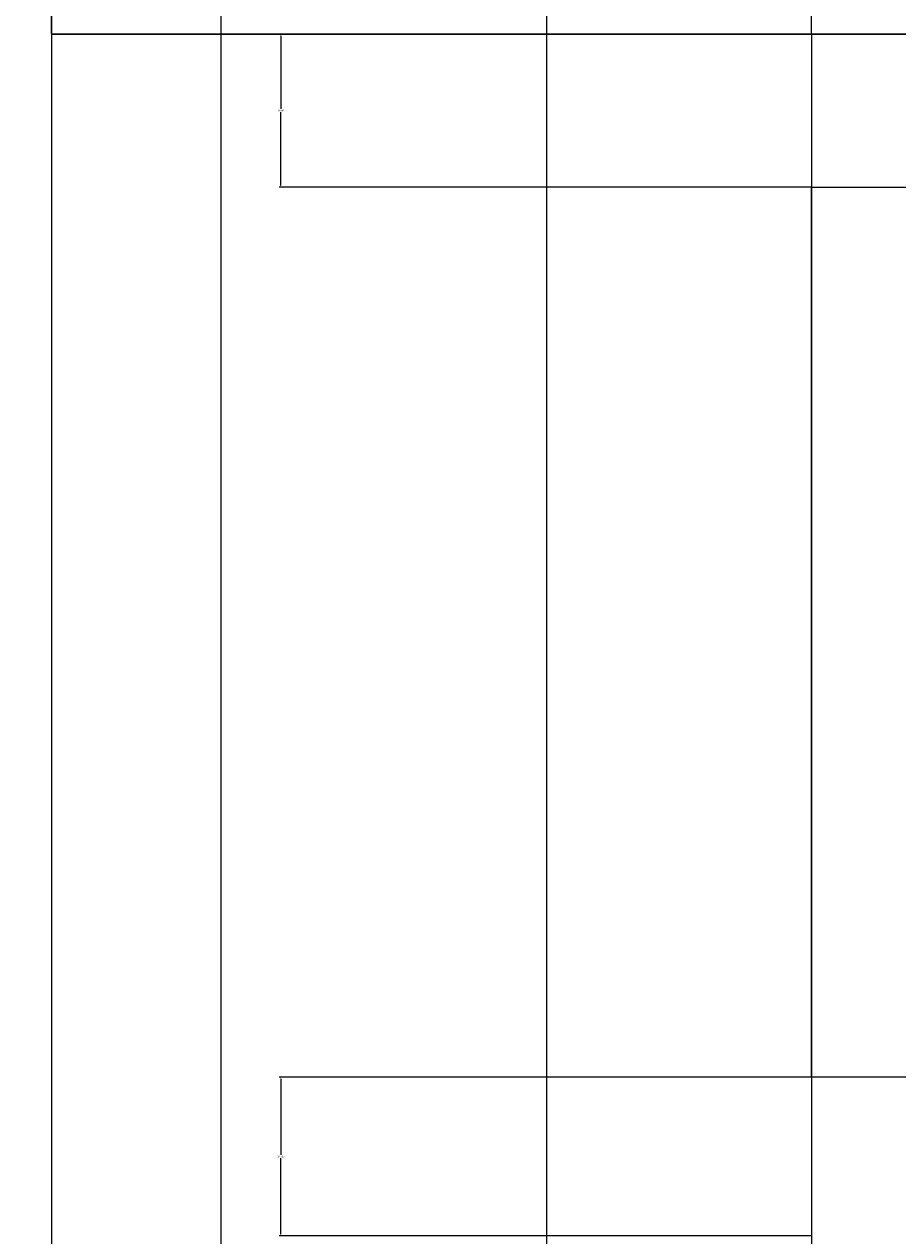
# Model space of a CAD drawing. Units: inches. Extents: x -46 to 1145, y -527 to 760.
# Tile 10 of 57: x 187 to 283, y -172 to -38. Entities that reach past the tile are written whole.
import ezdxf

# ---------------------------------------------------------------- set-up
doc = ezdxf.new("R2010")
doc.units = ezdxf.units.IN
doc.header["$MEASUREMENT"] = 0
for name, color, linetype, lineweight in [('A-ANNO-DIMS', 2, 'Continuous', 18), ('C-PKNG', 8, 'Continuous', 18), ('C-ROAD', 9, 'Continuous', 18), ('C-SITE', 7, 'Continuous', 30)]:
    doc.layers.add(name, color=color, linetype=linetype, lineweight=lineweight)
doc.styles.get("Standard").update_dxf_attribs({"font": 'arial.ttf'})
doc.dimstyles.get("Standard").update_dxf_attribs({"dimtxt": 0.18, "dimasz": 0.18, "dimexe": 0.18, "dimexo": 0.0625, "dimgap": 0.09, "dimtad": 0, "dimtih": 1, "dimtoh": 1, "dimdec": 0, "dimzin": 0, "dimdsep": 46, "dimlunit": 3, "dimtxsty": 'Standard', "dimcen": 0.09, "dimadec": 0, "dimazin": 0, "dimtfac": 1, "dimtdec": 0, "dimtofl": 0, "dimtmove": 0, "dimatfit": 3, "dimfxl": 1, "dimtolj": 1, "dimtzin": 0, "dimarcsym": 0})

# ---------------------------------------------------------------- blocks, each defined once
blk = doc.blocks.new('*D693')
at = {"layer": 'A-ANNO-DIMS', "color": 0, "lineweight": -2, "transparency": 16777216}
for p, q in [((189.56, -39.42), (189.56, 19.3)), ((189.74, 19.12), (231.15, 19.12)), ((273.34, 19.12), (231.93, 19.12)), ((273.52, -39.42), (273.52, 19.3))]:
    blk.add_line(p, q, dxfattribs=at)
at = {"layer": 'A-ANNO-DIMS', "color": 0, "transparency": 16777216}
for points in [[(189.74, 19.15), (189.74, 19.09), (189.56, 19.12)], [(273.34, 19.15), (273.34, 19.09), (273.52, 19.12)]]:
    blk.add_solid(points, dxfattribs=at)
at = {"layer": 'Defpoints', "color": 0, "transparency": 16777216}
for p in [(273.52, 19.12), (189.56, -39.48), (273.52, -39.48)]:
    blk.add_point(p, dxfattribs=at)
at = {"layer": 'A-ANNO-DIMS', "color": 0, "transparency": 16777216, "insert": (231.54, 19.12), "char_height": 0.18, "attachment_point": 5}
blk.add_mtext('\\A1;83.95', dxfattribs=at)
blk = doc.blocks.new('*D695')
at = {"layer": 'A-ANNO-DIMS', "color": 0, "lineweight": -2, "transparency": 16777216}
for p, q in [((208.27, 221.46), (208.27, -527.26)), ((244.27, 221.46), (244.27, -527.26)), ((208.45, -527.08), (226.05, -527.08)), ((244.09, -527.08), (226.49, -527.08))]:
    blk.add_line(p, q, dxfattribs=at)
at = {"layer": 'A-ANNO-DIMS', "color": 0, "transparency": 16777216}
for points in [[(208.45, -527.05), (208.45, -527.11), (208.27, -527.08)], [(244.09, -527.05), (244.09, -527.11), (244.27, -527.08)]]:
    blk.add_solid(points, dxfattribs=at)
at = {"layer": 'Defpoints', "color": 0, "transparency": 16777216}
for p in [(208.27, 221.52), (244.27, 221.52), (244.27, -527.08)]:
    blk.add_point(p, dxfattribs=at)
at = {"layer": 'A-ANNO-DIMS', "color": 0, "transparency": 16777216, "insert": (226.27, -527.08), "char_height": 0.18, "attachment_point": 5}
blk.add_mtext('\\A1;36', dxfattribs=at)
blk = doc.blocks.new('*D701')
at = {"layer": 'A-ANNO-DIMS', "color": 0, "lineweight": -2, "transparency": 16777216}
for p, q in [((273.45, -154.67), (214.74, -154.67)), ((214.92, -154.85), (214.92, -163.24)), ((214.92, -172), (214.92, -163.61)), ((273.45, -172.18), (214.74, -172.18))]:
    blk.add_line(p, q, dxfattribs=at)
at = {"layer": 'A-ANNO-DIMS', "color": 0, "transparency": 16777216}
for points in [[(214.89, -154.85), (214.95, -154.85), (214.92, -154.67)], [(214.89, -172), (214.95, -172), (214.92, -172.18)]]:
    blk.add_solid(points, dxfattribs=at)
at = {"layer": 'Defpoints', "color": 0, "transparency": 16777216}
for p in [(214.92, -154.67), (273.52, -154.67), (273.52, -172.18)]:
    blk.add_point(p, dxfattribs=at)
at = {"layer": 'A-ANNO-DIMS', "color": 0, "transparency": 16777216, "insert": (214.92, -163.42), "char_height": 0.18, "attachment_point": 5}
blk.add_mtext('\\A1;17.513', dxfattribs=at)
blk = doc.blocks.new('*D702')
at = {"layer": 'A-ANNO-DIMS', "color": 0, "lineweight": -2, "transparency": 16777216}
for p, q in [((189.63, -39.48), (1145.34, -39.48)), ((1145.16, -39.66), (1145.16, -249.3)), ((1145.16, -459.3), (1145.16, -249.66)), ((183.63, -459.48), (1145.34, -459.48))]:
    blk.add_line(p, q, dxfattribs=at)
at = {"layer": 'A-ANNO-DIMS', "color": 0, "transparency": 16777216}
for points in [[(1145.13, -39.66), (1145.19, -39.66), (1145.16, -39.48)], [(1145.13, -459.3), (1145.19, -459.3), (1145.16, -459.48)]]:
    blk.add_solid(points, dxfattribs=at)
at = {"layer": 'Defpoints', "color": 0, "transparency": 16777216}
for p in [(189.56, -39.48), (1145.16, -39.48), (183.56, -459.48)]:
    blk.add_point(p, dxfattribs=at)
at = {"layer": 'A-ANNO-DIMS', "color": 0, "transparency": 16777216, "insert": (1145.16, -249.48), "char_height": 0.18, "attachment_point": 5}
blk.add_mtext('\\A1;420', dxfattribs=at)
blk = doc.blocks.new('*D703')
at = {"layer": 'A-ANNO-DIMS', "color": 0, "lineweight": -2, "transparency": 16777216}
for p, q in [((273.45, -39.48), (214.74, -39.48)), ((214.92, -39.66), (214.92, -47.74)), ((214.92, -56.19), (214.92, -48.11)), ((273.45, -56.37), (214.74, -56.37))]:
    blk.add_line(p, q, dxfattribs=at)
at = {"layer": 'A-ANNO-DIMS', "color": 0, "transparency": 16777216}
for points in [[(214.89, -39.66), (214.95, -39.66), (214.92, -39.48)], [(214.89, -56.19), (214.95, -56.19), (214.92, -56.37)]]:
    blk.add_solid(points, dxfattribs=at)
at = {"layer": 'Defpoints', "color": 0, "transparency": 16777216}
for p in [(214.92, -39.48), (273.52, -39.48), (273.52, -56.37)]:
    blk.add_point(p, dxfattribs=at)
at = {"layer": 'A-ANNO-DIMS', "color": 0, "transparency": 16777216, "insert": (214.92, -47.93), "char_height": 0.18, "attachment_point": 5}
blk.add_mtext('\\A1;16.888', dxfattribs=at)

msp = doc.modelspace()

# ---------------------------------------------------------------- linework, layer by layer
at = {"layer": 'C-PKNG'}
msp.add_line((273.5156, -39.4824), (273.5156, -459.4824), dxfattribs=at)
msp.add_lwpolyline([(501.7297, -154.6684), (273.5156, -154.6684), (273.5156, -56.3706), (501.7297, -56.3706)], close=True, dxfattribs=at)
at = {"layer": 'C-ROAD'}
msp.add_line((189.5637, 221.5176), (189.5637, -468.4824), dxfattribs=at)
at = {"layer": 'C-SITE'}
msp.add_line((590.0637, -39.4824), (189.5637, -39.4824), dxfattribs=at)

# ---------------------------------------------------------------- dimensions: what is measured, and where the dimension line sits
at = {"layer": 'A-ANNO-DIMS'}
for base, p1, p2, override, picture, middle in [((244.2731, -527.0824), (208.2731, 221.5176), (244.2731, 221.5176), {"dimdec": 0, "dimlfac": 1, "dimrnd": 0, "dimzin": 0, "dimdsep": 46, "dimlunit": 2}, '*D695', (226.2731, -527.0824)), ((273.5156, 19.1176), (189.5637, -39.4824), (273.5156, -39.4824), {"dimdec": 2, "dimlfac": 1, "dimrnd": 0, "dimzin": 0, "dimdsep": 46, "dimlunit": 2}, '*D693', (231.5397, 19.1176))]:
    dim = msp.add_linear_dim(base=base, p1=p1, p2=p2, dimstyle='Standard', override=override, dxfattribs=at)
    dim.commit()
    dim.dimension.update_dxf_attribs({"geometry": picture, "text_midpoint": middle})
for base, p1, p2, override, picture, middle in [((1145.1637, -39.4824), (183.5637, -459.4824), (189.5637, -39.4824), {"dimdec": 0, "dimlfac": 1, "dimrnd": 0, "dimzin": 0, "dimdsep": 46, "dimlunit": 2}, '*D702', (1145.1637, -249.4824)), ((214.9156, -39.4824), (273.5156, -56.3706), (273.5156, -39.4824), {"dimdec": 3, "dimlfac": 1, "dimrnd": 0, "dimzin": 0, "dimdsep": 46, "dimlunit": 2}, '*D703', (214.9156, -47.9265)), ((214.9156, -154.6684), (273.5156, -172.1813), (273.5156, -154.6684), {"dimdec": 3, "dimlfac": 1, "dimrnd": 0, "dimzin": 0, "dimdsep": 46, "dimlunit": 2}, '*D701', (214.9156, -163.4249))]:
    dim = msp.add_linear_dim(base=base, p1=p1, p2=p2, angle=90, dimstyle='Standard', override=override, dxfattribs=at)
    dim.commit()
    dim.dimension.update_dxf_attribs({"geometry": picture, "text_midpoint": middle})

doc.saveas('drawing.dxf')
